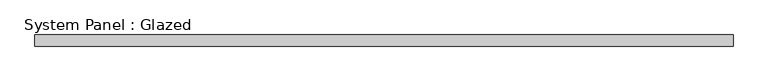
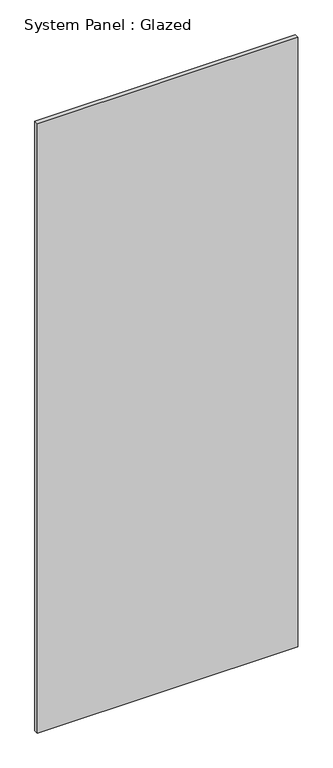
"""IFC4 building model written with IfcOpenShell, lengths in millimetres: plate geometry, System Panel : Glazed."""

from ifc_helpers import new_model, si_unit, origin, origin_with_axes, place, context, project, spatial, polyline, outline, extrude, source, transform, mapped, element, save


def system_panel_glazed_62c681ce(model_context):
    return source(origin(), model_context, "Body", "SweptSolid", [
        extrude(outline(polyline([(774.7, 19.05), (-774.7, 19.05), (-774.7, 44.45), (774.7, 44.45), (774.7, 19.05)])), origin_with_axes(), (0.0, 0.0, 1.0), 3835.4),
    ])


if __name__ == "__main__":
    model = new_model("IFC4")
    model_context = context("Model", 3, world=origin())
    ifc_project = project(units=[si_unit("LENGTHUNIT", "METRE", prefix="MILLI")], contexts=[model_context])
    site = spatial("IfcSite", under=ifc_project)
    building = spatial("IfcBuilding", under=site)
    placement = place(None, origin())
    system_panel_glazed_shape = system_panel_glazed_62c681ce(model_context)
    element("IfcPlate", 1, ObjectType="System Panel : Glazed", at=placement, inside=building, context=model_context, shape_type="MappedRepresentation", body=[
        mapped(system_panel_glazed_shape, transform((0.0, 0.0, 0.0), x_axis=(1.0, 0.0, 0.0), y_axis=(0.0, 1.0, 0.0), z_axis=(0.0, 0.0, 1.0))),
    ])
    save(model, "model.ifc")

# Revit data of these elements
# Type "System Panel : Glazed"
#   Construction Type Id = "GSP4R"
#   Analytic Construction = "1/8 in Pilkington single glazing"
#   Visual Light Transmittance = 0.9
#   Solar Heat Gain Coefficient = 0.86
#   Heat Transfer Coefficient (U) = 1.18115 BTU/(h·ft²·°F)
# Element 1 (IfcPlate, "System Panel : Glazed")
#   Materials on its faces: "Glass"
# Materials
#   "Glass": class "Glass", colour RGB 0 128 192, transparency 0.75, Description = "Soda Lime Glass", Cost = 0
